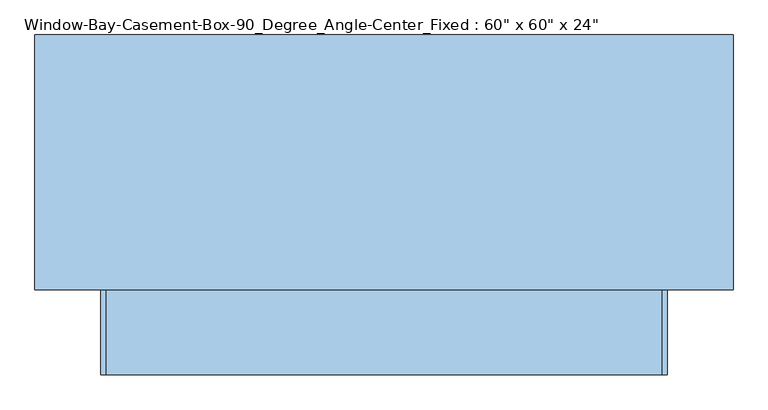
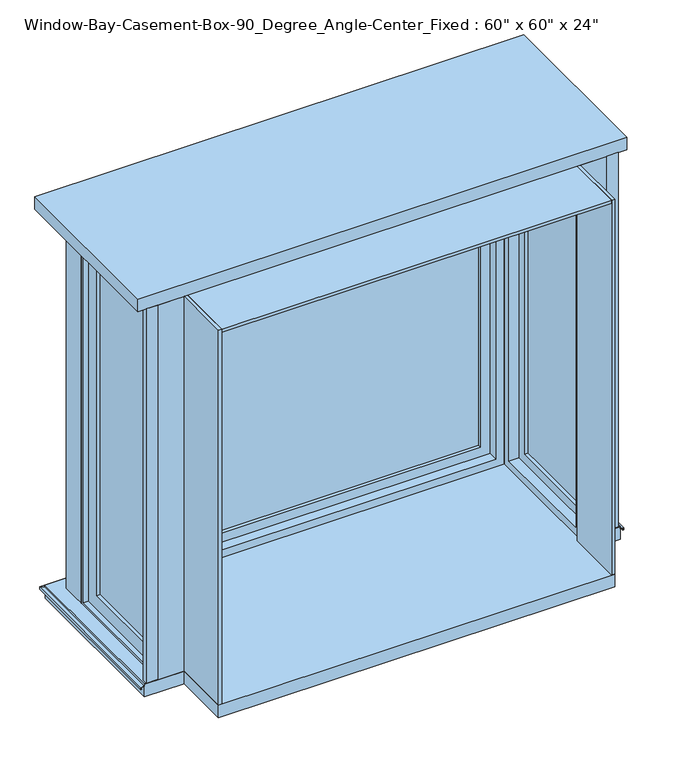
"""IFC4 building model written with IfcOpenShell, lengths in millimetres: window geometry."""

from ifc_helpers import new_model, si_unit, frame, origin, place, context, project, spatial, polyline, outline, extrude, faceted_brep, source, transform, mapped, element, save


def window_dda79932(model_context):
    return source(origin(), model_context, "Body", "SolidModel", [
        extrude(outline(polyline([(-863.6, 114.3), (-908.05, 114.3), (-908.05, 133.35), (-863.6, 133.35), (-863.6, 114.3)])), frame((0.0, 0.0, 663.1486341), z_axis=(0.0, 0.0, 1.0), x_axis=(1.0, 0.0, 0.0)), (0.0, 0.0, 1.0), 1521.2513659),
        extrude(outline(polyline([(908.05, 114.3), (863.6, 114.3), (863.6, 133.35), (908.05, 133.35), (908.05, 114.3)])), frame((0.0, 0.0, 663.1486341), z_axis=(0.0, 0.0, 1.0), x_axis=(1.0, 0.0, 0.0)), (0.0, 0.0, 1.0), 1521.2513659),
        faceted_brep([(-914.4, 114.3, 653.0697935), (-914.4, 114.3, 660.4), (-863.6, 114.3, 660.4), (-863.6, 114.3, 663.1486341), (-915.797, 114.3, 663.1486341), (-915.797, 114.3, 654.4483503), (-928.497, 114.3, 652.2089977), (-928.497, 114.3, 643.2668038), (-924.5346, 114.3, 643.2668038), (-924.5346, 114.3, 644.7270038), (-926.8968, 114.3, 644.7270038), (-926.8968, 114.3, 650.8662705), (914.4, 114.3, 653.0697935), (926.8968, 114.3, 650.8662705), (926.8968, 114.3, 644.7270038), (924.5346, 114.3, 644.7270038), (924.5346, 114.3, 643.2668038), (928.497, 114.3, 643.2668038), (928.497, 114.3, 652.2089977), (915.797, 114.3, 654.4483503), (915.797, 114.3, 663.1486341), (863.6, 114.3, 663.1486341), (863.6, 114.3, 660.4), (914.4, 114.3, 660.4), (-914.4, 774.7, 653.0697935), (-914.4, 774.7, 660.4), (914.4, 774.7, 660.4), (863.6, 723.9, 660.4), (-863.6, 723.9, 660.4), (-863.6, 723.9, 663.1486341), (863.6, 723.9, 663.1486341), (915.797, 776.097, 663.1486341), (-915.797, 776.097, 663.1486341), (-915.797, 776.097, 654.4483503), (-928.497, 788.797, 652.2089977), (-928.497, 788.797, 643.2668038), (928.497, 788.797, 643.2668038), (924.5346, 784.8346, 643.2668038), (-924.5346, 784.8346, 643.2668038), (-924.5346, 784.8346, 644.7270038), (924.5346, 784.8346, 644.7270038), (926.8968, 787.1968, 644.7270038), (-926.8968, 787.1968, 644.7270038), (-926.8968, 787.1968, 650.8662705), (914.4, 774.7, 653.0697935), (915.797, 776.097, 654.4483503), (928.497, 788.797, 652.2089977), (926.8968, 787.1968, 650.8662705)], [[[0, 1, 2, 3, 4, 5, 6, 7, 8, 9, 10, 11]], [[12, 13, 14, 15, 16, 17, 18, 19, 20, 21, 22, 23]], [[1, 0, 24, 25]], [[2, 1, 25, 26, 23, 22, 27, 28]], [[3, 2, 28, 29]], [[4, 3, 29, 30, 21, 20, 31, 32]], [[5, 4, 32, 33]], [[6, 5, 33, 34]], [[7, 6, 34, 35]], [[8, 7, 35, 36, 17, 16, 37, 38]], [[9, 8, 38, 39]], [[10, 9, 39, 40, 15, 14, 41, 42]], [[11, 10, 42, 43]], [[0, 11, 43, 24]], [[25, 24, 44, 26]], [[29, 28, 27, 30]], [[33, 32, 31, 45]], [[34, 33, 45, 46]], [[35, 34, 46, 36]], [[39, 38, 37, 40]], [[43, 42, 41, 47]], [[24, 43, 47, 44]], [[26, 44, 12, 23]], [[30, 27, 22, 21]], [[45, 31, 20, 19]], [[46, 45, 19, 18]], [[36, 46, 18, 17]], [[40, 37, 16, 15]], [[47, 41, 14, 13]], [[44, 47, 13, 12]]]),
        extrude(outline(polyline([(914.4, 774.7), (914.4, 114.3), (762.0, 114.3), (762.0, -114.3), (-762.0, -114.3), (-762.0, 114.3), (-914.4, 114.3), (-914.4, 774.7), (914.4, 774.7)])), frame((0.0, 0.0, 609.6), z_axis=(0.0, 0.0, 1.0), x_axis=(1.0, 0.0, 0.0)), (0.0, 0.0, 1.0), 50.8),
        extrude(outline(polyline([(939.8, 800.1), (939.8, 114.3), (-939.8, 114.3), (-939.8, 800.1), (939.8, 800.1)])), frame((0.0, 0.0, 2184.4), z_axis=(0.0, 0.0, 1.0), x_axis=(1.0, 0.0, 0.0)), (0.0, 0.0, 1.0), 50.8),
        extrude(outline(polyline([(-762.0, 723.9), (-762.0, 622.3), (-863.6, 622.3), (-863.6, 723.9), (-762.0, 723.9)])), frame((0.0, 0.0, 660.4), z_axis=(0.0, 0.0, 1.0), x_axis=(1.0, 0.0, 0.0)), (0.0, 0.0, 1.0), 1524.0),
        extrude(outline(polyline([(863.6, 723.9), (863.6, 622.3), (762.0, 622.3), (762.0, 723.9), (863.6, 723.9)])), frame((0.0, 0.0, 660.4), z_axis=(0.0, 0.0, 1.0), x_axis=(1.0, 0.0, 0.0)), (0.0, 0.0, 1.0), 1524.0),
        faceted_brep([(749.3, 660.4, 673.1), (749.3, 723.9, 673.1), (-749.3, 723.9, 673.1), (-749.3, 660.4, 673.1), (730.25, 622.3, 692.15), (730.25, 660.4, 692.15), (-730.25, 660.4, 692.15), (-730.25, 622.3, 692.15), (762.0, 723.9, 660.4), (762.0, 622.3, 660.4), (-762.0, 622.3, 660.4), (-762.0, 723.9, 660.4), (-749.3, 723.9, 2171.7), (-749.3, 660.4, 2171.7), (-730.25, 660.4, 2152.65), (-730.25, 622.3, 2152.65), (-762.0, 622.3, 2184.4), (-762.0, 723.9, 2184.4), (749.3, 723.9, 2171.7), (749.3, 660.4, 2171.7), (730.25, 660.4, 2152.65), (730.25, 622.3, 2152.65), (762.0, 622.3, 2184.4), (762.0, 723.9, 2184.4)], [[[0, 1, 2, 3]], [[4, 5, 6, 7]], [[8, 9, 10, 11]], [[3, 2, 12, 13]], [[7, 6, 14, 15]], [[11, 10, 16, 17]], [[13, 12, 18, 19]], [[15, 14, 20, 21]], [[17, 16, 22, 23]], [[11, 17, 23, 8], [1, 18, 12, 2]], [[19, 18, 1, 0]], [[3, 13, 19, 0], [5, 20, 14, 6]], [[21, 20, 5, 4]], [[9, 22, 16, 10], [7, 15, 21, 4]], [[23, 22, 9, 8]]]),
        extrude(outline(polyline([(2171.7, -749.3), (673.1, -749.3), (673.1, 749.3), (2171.7, 749.3), (2171.7, -749.3)]), holes=[polyline([(2114.55, 692.15), (730.25, 692.15), (730.25, -692.15), (2114.55, -692.15), (2114.55, 692.15)])]), frame((0.0, 660.4, 0.0), z_axis=(0.0, 1.0, 0.0), x_axis=(0.0, 0.0, 1.0)), (0.0, 0.0, 1.0), 44.45),
        faceted_brep([(-762.0, 146.05, 2152.65), (-800.1, 146.05, 2152.65), (-800.1, 590.55, 2152.65), (-762.0, 590.55, 2152.65), (-863.6, 114.3, 2184.4), (-762.0, 114.3, 2184.4), (-762.0, 622.3, 2184.4), (-863.6, 622.3, 2184.4), (-800.1, 127.0, 2171.7), (-863.6, 127.0, 2171.7), (-863.6, 609.6, 2171.7), (-800.1, 609.6, 2171.7), (-800.1, 590.55, 692.15), (-762.0, 590.55, 692.15), (-762.0, 622.3, 660.4), (-863.6, 622.3, 660.4), (-863.6, 609.6, 673.1), (-800.1, 609.6, 673.1), (-800.1, 146.05, 692.15), (-762.0, 146.05, 692.15), (-762.0, 114.3, 660.4), (-863.6, 114.3, 660.4), (-863.6, 127.0, 673.1), (-800.1, 127.0, 673.1)], [[[0, 1, 2, 3]], [[4, 5, 6, 7]], [[8, 9, 10, 11]], [[3, 2, 12, 13]], [[7, 6, 14, 15]], [[11, 10, 16, 17]], [[13, 12, 18, 19]], [[15, 14, 20, 21]], [[17, 16, 22, 23]], [[11, 17, 23, 8], [1, 18, 12, 2]], [[19, 18, 1, 0]], [[5, 20, 14, 6], [3, 13, 19, 0]], [[21, 20, 5, 4]], [[7, 15, 21, 4], [9, 22, 16, 10]], [[23, 22, 9, 8]]]),
        extrude(outline(polyline([(609.6, 2171.7), (609.6, 673.1), (127.0, 673.1), (127.0, 2171.7), (609.6, 2171.7)]), holes=[polyline([(184.15, 2114.55), (184.15, 730.25), (552.45, 730.25), (552.45, 2114.55), (184.15, 2114.55)])]), frame((-844.55, 0.0, 0.0), z_axis=(1.0, 0.0, 0.0), x_axis=(0.0, 1.0, 0.0)), (0.0, 0.0, 1.0), 44.45),
        faceted_brep([(800.1, 146.05, 2152.65), (762.0, 146.05, 2152.65), (762.0, 590.55, 2152.65), (800.1, 590.55, 2152.65), (863.6, 127.0, 2171.7), (800.1, 127.0, 2171.7), (800.1, 609.6, 2171.7), (863.6, 609.6, 2171.7), (762.0, 114.3, 2184.4), (863.6, 114.3, 2184.4), (863.6, 622.3, 2184.4), (762.0, 622.3, 2184.4), (762.0, 590.55, 692.15), (800.1, 590.55, 692.15), (800.1, 609.6, 673.1), (863.6, 609.6, 673.1), (863.6, 622.3, 660.4), (762.0, 622.3, 660.4), (762.0, 146.05, 692.15), (800.1, 146.05, 692.15), (800.1, 127.0, 673.1), (863.6, 127.0, 673.1), (863.6, 114.3, 660.4), (762.0, 114.3, 660.4)], [[[0, 1, 2, 3]], [[4, 5, 6, 7]], [[8, 9, 10, 11]], [[3, 2, 12, 13]], [[7, 6, 14, 15]], [[11, 10, 16, 17]], [[13, 12, 18, 19]], [[15, 14, 20, 21]], [[17, 16, 22, 23]], [[11, 17, 23, 8], [1, 18, 12, 2]], [[19, 18, 1, 0]], [[5, 20, 14, 6], [3, 13, 19, 0]], [[21, 20, 5, 4]], [[9, 22, 16, 10], [7, 15, 21, 4]], [[23, 22, 9, 8]]]),
        extrude(outline(polyline([(609.6, 2171.7), (609.6, 673.1), (127.0, 673.1), (127.0, 2171.7), (609.6, 2171.7)]), holes=[polyline([(184.15, 2114.55), (184.15, 730.25), (552.45, 730.25), (552.45, 2114.55), (184.15, 2114.55)])]), frame((800.1, 0.0, 0.0), z_axis=(1.0, 0.0, 0.0), x_axis=(0.0, 1.0, 0.0)), (0.0, 0.0, 1.0), 44.45),
        extrude(outline(polyline([(692.15, 692.15), (692.15, 685.8), (-692.15, 685.8), (-692.15, 692.15), (692.15, 692.15)])), frame((0.0, 0.0, 730.25), z_axis=(0.0, 0.0, 1.0), x_axis=(1.0, 0.0, 0.0)), (0.0, 0.0, 1.0), 1384.3),
        extrude(outline(polyline([(692.15, 679.45), (692.15, 673.1), (-692.15, 673.1), (-692.15, 679.45), (692.15, 679.45)])), frame((0.0, 0.0, 730.25), z_axis=(0.0, 0.0, 1.0), x_axis=(1.0, 0.0, 0.0)), (0.0, 0.0, 1.0), 1384.3),
        extrude(outline(polyline([(-825.5, 552.45), (-825.5, 184.15), (-831.85, 184.15), (-831.85, 552.45), (-825.5, 552.45)])), frame((0.0, 0.0, 730.25), z_axis=(0.0, 0.0, 1.0), x_axis=(1.0, 0.0, 0.0)), (0.0, 0.0, 1.0), 1384.3),
        extrude(outline(polyline([(-812.8, 552.45), (-812.8, 184.15), (-819.15, 184.15), (-819.15, 552.45), (-812.8, 552.45)])), frame((0.0, 0.0, 730.25), z_axis=(0.0, 0.0, 1.0), x_axis=(1.0, 0.0, 0.0)), (0.0, 0.0, 1.0), 1384.3),
        extrude(outline(polyline([(831.85, 552.45), (831.85, 184.15), (825.5, 184.15), (825.5, 552.45), (831.85, 552.45)])), frame((0.0, 0.0, 730.25), z_axis=(0.0, 0.0, 1.0), x_axis=(1.0, 0.0, 0.0)), (0.0, 0.0, 1.0), 1384.3),
        extrude(outline(polyline([(819.15, 552.45), (819.15, 184.15), (812.8, 184.15), (812.8, 552.45), (819.15, 552.45)])), frame((0.0, 0.0, 730.25), z_axis=(0.0, 0.0, 1.0), x_axis=(1.0, 0.0, 0.0)), (0.0, 0.0, 1.0), 1384.3),
        faceted_brep([(863.6, 127.0, 2171.7), (800.1, 127.0, 2171.7), (800.1, 609.6, 2171.7), (863.6, 609.6, 2171.7), (762.0, 114.3, 2184.4), (863.6, 114.3, 2184.4), (863.6, 622.3, 2184.4), (762.0, 622.3, 2184.4), (800.1, 146.05, 2152.65), (762.0, 146.05, 2152.65), (762.0, 590.55, 2152.65), (800.1, 590.55, 2152.65), (800.1, 609.6, 673.1), (863.6, 609.6, 673.1), (863.6, 622.3, 660.4), (762.0, 622.3, 660.4), (762.0, 590.55, 692.15), (800.1, 590.55, 692.15), (800.1, 127.0, 673.1), (863.6, 127.0, 673.1), (863.6, 114.3, 660.4), (762.0, 114.3, 660.4), (762.0, 146.05, 692.15), (800.1, 146.05, 692.15)], [[[0, 1, 2, 3]], [[4, 5, 6, 7]], [[8, 9, 10, 11]], [[3, 2, 12, 13]], [[7, 6, 14, 15]], [[11, 10, 16, 17]], [[13, 12, 18, 19]], [[15, 14, 20, 21]], [[17, 16, 22, 23]], [[1, 18, 12, 2], [11, 17, 23, 8]], [[19, 18, 1, 0]], [[5, 20, 14, 6], [3, 13, 19, 0]], [[21, 20, 5, 4]], [[7, 15, 21, 4], [9, 22, 16, 10]], [[23, 22, 9, 8]]]),
        extrude(outline(polyline([(-749.3, 114.3), (-749.3, -114.3), (-762.0, -114.3), (-762.0, 114.3), (-749.3, 114.3)])), frame((0.0, 0.0, 660.4), z_axis=(0.0, 0.0, 1.0), x_axis=(1.0, 0.0, 0.0)), (0.0, 0.0, 1.0), 1524.0),
        extrude(outline(polyline([(749.3, 114.3), (762.0, 114.3), (762.0, -114.3), (749.3, -114.3), (749.3, 114.3)])), frame((0.0, 0.0, 660.4), z_axis=(0.0, 0.0, 1.0), x_axis=(1.0, 0.0, 0.0)), (0.0, 0.0, 1.0), 1524.0),
        extrude(outline(polyline([(749.3, -114.3), (-749.3, -114.3), (-749.3, 622.3), (749.3, 622.3), (749.3, -114.3)])), frame((0.0, 0.0, 2171.7), z_axis=(0.0, 0.0, 1.0), x_axis=(1.0, 0.0, 0.0)), (0.0, 0.0, 1.0), 12.7),
    ])


if __name__ == "__main__":
    model = new_model("IFC4")
    model_context = context("Model", 3, world=origin())
    ifc_project = project(units=[si_unit("LENGTHUNIT", "METRE", prefix="MILLI")], contexts=[model_context])
    site = spatial("IfcSite", under=ifc_project)
    building = spatial("IfcBuilding", under=site)
    placement = place(None, origin())
    window_shape = window_dda79932(model_context)
    element("IfcWindow", 1, ObjectType="Window-Bay-Casement-Box-90_Degree_Angle-Center_Fixed : 60\" x 60\" x 24\"", at=placement, inside=building, context=model_context, shape_type="MappedRepresentation", body=[
        mapped(window_shape, transform((0.0, 0.0, 0.0), x_axis=(1.0, 0.0, 0.0), y_axis=(0.0, 1.0, 0.0), z_axis=(0.0, 0.0, 1.0))),
    ])
    save(model, "model.ifc")

# Revit data of these elements
# Type "Window-Bay-Casement-Box-90_Degree_Angle-Center_Fixed : 60\" x 60\" x 24\""
#   Type Mark = "18"
#   Fire Rating = "0.5h"
#   Assembly Code = "B2020100"
#   Analytic Construction = "1/8 in Pilkington single glazing"
#   Width = 5' - 0"
#   Wall Thickness [instance default] = 0' - 6"
#   Visual Light Transmittance = 0.9
#   Trim Width = 5' - 8"
#   Trim Height = 5' - 0"
#   Thermal Resistance (R) = 1.5394 (h·ft²·°F)/BTU
#   Solar Heat Gain Coefficient = 0.86
#   Rough Width = 5' - 0 1/2"
#   Rough Height = 5' - 0 1/2"
#   Height 1 = 5' - 2"
#   Height = 5' - 0"
#   Heat Transfer Coefficient (U) = 0.6496 BTU/(h·ft²·°F)
#   Depth = 2' - 0"
#   Default Sill Height = 2' - 0"
#   Side Muntin Visibility = yes
#   Center Muntin Visibility = yes
#   Interior Trim Visibility [instance default] = yes
#   Exterior Trim Visibility [instance default] = yes
#   Side Muntin Pattern = Muntin Pattern_2x2 : Muntin Pattern_2x2
#   Center Muntin Pattern = Muntin Pattern_2x2 : Muntin Pattern_2x2
#   Interior Trim Material = Wood - Stained
#   Exterior Trim Material = Clad - White
#   Exterior Trim = element 385931
#   Interior Trim = Trim-Window-Interior-Flat : Picture Frame
#   Interior Frame Material = Wood - Stained
#   Glass Panel Material = Glass
#   Exterior Frame Material = Clad - White
#   Wall Closure = (empty or 0)
# Element 1 (IfcWindow, "Window-Bay-Casement-Box-90_Degree_Angle-Center_Fixed : 60\" x 60\" x 24\"")
#   Wall Thickness = 0' - 9"
#   Materials on its faces: "Clad - White", "Wood - Stained", "Glass"
# Materials
#   "Wood - Stained": class "Wood", colour RGB 224 178 126, transparency 0, Cost = 0
#   "Clad - White": class "Wood", colour RGB 242 242 238, transparency 0, Cost = 0
#   "Glass": class "Glass", colour RGB 0 128 192, transparency 0.75, Description = "Soda Lime Glass", Cost = 0
